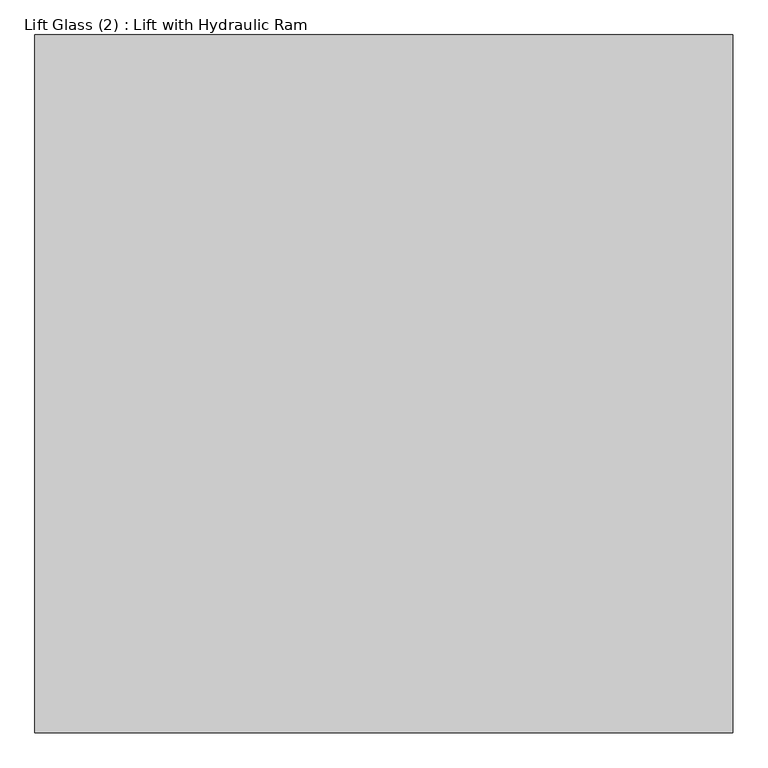
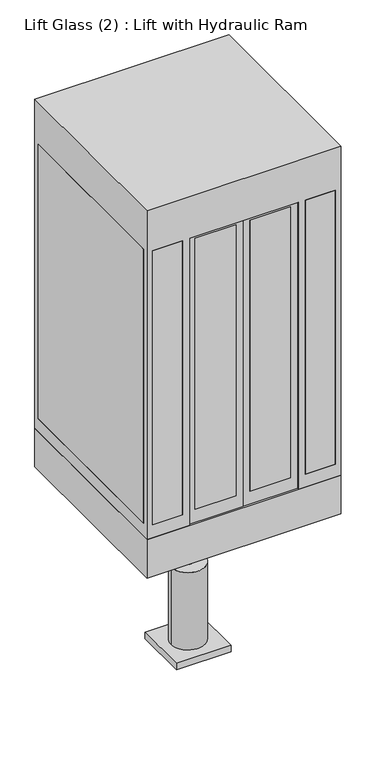
"""IFC4 building model written with IfcOpenShell, lengths in millimetres: proxy geometry, Lift Glass (2) : Lift with Hydraulic Ram."""

from ifc_helpers import new_model, si_unit, point, frame, frame_2d, origin, place, context, project, spatial, polyline, circle_curve, trimmed, segment, composite_curve, outline, extrude, faceted_brep, source, transform, mapped, element, save


def lift_glass_2_lift_with_hydraulic_ram_a28bd677(model_context):
    return source(origin(), model_context, "Body", "SolidModel", [
        extrude(outline(composite_curve([segment(trimmed(circle_curve(frame_2d((34.4858536, 51.9253128)), 35.0), [point((34.4858536, 86.9253128))], [point((34.4858536, 16.9253128))], False, "CARTESIAN"), True, "CONTINUOUS"), segment(trimmed(circle_curve(frame_2d((34.4858536, 51.9253128)), 35.0), [point((34.4858536, 16.9253128))], [point((34.4858536, 86.9253128))], False, "CARTESIAN"), True, "CONTINUOUS")], self_intersect=False)), frame((0.0, 0.0, -850.0), z_axis=(0.0, 0.0, 1.0), x_axis=(1.0, 0.0, 0.0)), (0.0, 0.0, 1.0), 550.0),
        extrude(outline(composite_curve([segment(trimmed(circle_curve(frame_2d((34.4858536, 51.9253128)), 125.0), [point((-90.5141464, 51.9253128))], [point((159.4858536, 51.9253128))], False, "CARTESIAN"), True, "CONTINUOUS"), segment(trimmed(circle_curve(frame_2d((34.4858536, 51.9253128)), 125.0), [point((159.4858536, 51.9253128))], [point((-90.5141464, 51.9253128))], False, "CARTESIAN"), True, "CONTINUOUS")], self_intersect=False)), frame((0.0, 0.0, -1450.0), z_axis=(0.0, 0.0, 1.0), x_axis=(1.0, 0.0, 0.0)), (0.0, 0.0, 1.0), 600.0),
        extrude(outline(polyline([(234.4858536, -148.0746872), (-165.5141464, -148.0746872), (-165.5141464, 251.9253128), (234.4858536, 251.9253128), (234.4858536, -148.0746872)])), frame((0.0, 0.0, -1500.0), z_axis=(0.0, 0.0, 1.0), x_axis=(1.0, 0.0, 0.0)), (0.0, 0.0, 1.0), 50.0),
        extrude(outline(polyline([(-15.5141464, -648.0746872), (-315.5141464, -648.0746872), (-315.5141464, -636.0746872), (-15.5141464, -636.0746872), (-15.5141464, -648.0746872)])), frame((0.0, 0.0, 100.0), z_axis=(0.0, 0.0, 1.0), x_axis=(1.0, 0.0, 0.0)), (0.0, 0.0, 1.0), 2100.0),
        extrude(outline(polyline([(384.4858536, -648.0746872), (84.4858536, -648.0746872), (84.4858536, -636.0746872), (384.4858536, -636.0746872), (384.4858536, -648.0746872)])), frame((0.0, 0.0, 100.0), z_axis=(0.0, 0.0, 1.0), x_axis=(1.0, 0.0, 0.0)), (0.0, 0.0, 1.0), 2100.0),
        extrude(outline(polyline([(2300.0, 33.4858536), (2300.0, -365.5141464), (0.0, -365.5141464), (0.0, 33.4858536), (2300.0, 33.4858536)]), holes=[polyline([(2200.0, -15.5141464), (100.0, -15.5141464), (100.0, -315.5141464), (2200.0, -315.5141464), (2200.0, -15.5141464)])]), frame((0.0, -648.0746872, 0.0), z_axis=(0.0, 1.0, 0.0), x_axis=(0.0, 0.0, 1.0)), (0.0, 0.0, 1.0), 12.0),
        extrude(outline(polyline([(0.0, 35.4858536), (0.0, 434.4858536), (2300.0, 434.4858536), (2300.0, 35.4858536), (0.0, 35.4858536)]), holes=[polyline([(2200.0, 384.4858536), (100.0, 384.4858536), (100.0, 84.4858536), (2200.0, 84.4858536), (2200.0, 384.4858536)])]), frame((0.0, -648.0746872, 0.0), z_axis=(0.0, 1.0, 0.0), x_axis=(0.0, 0.0, 1.0)), (0.0, 0.0, 1.0), 12.0),
        extrude(outline(polyline([(746.4858536, 763.9253128), (746.4858536, -660.0746872), (-677.5141464, -660.0746872), (-677.5141464, 763.9253128), (746.4858536, 763.9253128)])), frame((0.0, 0.0, -300.0), z_axis=(0.0, 0.0, 1.0), x_axis=(1.0, 0.0, 0.0)), (0.0, 0.0, 1.0), 300.0),
        faceted_brep([(734.4858536, 721.9253128, 100.0), (734.4858536, -618.0746872, 100.0), (746.4858536, -618.0746872, 100.0), (746.4858536, 721.9253128, 100.0), (-665.5141464, -618.0746872, 100.0), (-665.5141464, 721.9253128, 100.0), (-677.5141464, 721.9253128, 100.0), (-677.5141464, -618.0746872, 100.0), (-635.5141464, 751.9253128, 100.0), (704.4858536, 751.9253128, 100.0), (704.4858536, 763.9253128, 100.0), (-635.5141464, 763.9253128, 100.0), (704.4858536, -660.0746872, 100.0), (704.4858536, -648.0746872, 100.0), (484.4858536, -648.0746872, 100.0), (484.4858536, -660.0746872, 100.0), (-635.5141464, -648.0746872, 100.0), (-635.5141464, -660.0746872, 100.0), (-415.5141464, -660.0746872, 100.0), (-415.5141464, -648.0746872, 100.0), (434.4858536, -660.0746872, 0.0), (434.4858536, -648.0746872, 0.0), (734.4858536, -648.0746872, 0.0), (734.4858536, 751.9253128, 0.0), (-665.5141464, 751.9253128, 0.0), (-665.5141464, -648.0746872, 0.0), (-365.5141464, -648.0746872, 0.0), (-365.5141464, -660.0746872, 0.0), (-677.5141464, -660.0746872, 0.0), (-677.5141464, 763.9253128, 0.0), (746.4858536, 763.9253128, 0.0), (746.4858536, -660.0746872, 0.0), (734.4858536, 751.9253128, 2300.0), (734.4858536, -648.0746872, 2300.0), (734.4858536, 721.9253128, 2225.0), (734.4858536, -618.0746872, 2225.0), (746.4858536, 763.9253128, 2550.0), (746.4858536, -660.0746872, 2550.0), (746.4858536, -618.0746872, 2225.0), (746.4858536, 721.9253128, 2225.0), (434.4858536, -660.0746872, 2225.0), (434.4858536, -648.0746872, 2225.0), (-677.5141464, -660.0746872, 2550.0), (-365.5141464, -660.0746872, 2225.0), (-635.5141464, -660.0746872, 2225.0), (-415.5141464, -660.0746872, 2225.0), (704.4858536, -660.0746872, 2225.0), (484.4858536, -660.0746872, 2225.0), (-365.5141464, -648.0746872, 2225.0), (-665.5141464, -648.0746872, 2300.0), (-635.5141464, -648.0746872, 2225.0), (-415.5141464, -648.0746872, 2225.0), (704.4858536, -648.0746872, 2225.0), (484.4858536, -648.0746872, 2225.0), (-665.5141464, 751.9253128, 2300.0), (-665.5141464, -618.0746872, 2225.0), (-665.5141464, 721.9253128, 2225.0), (-677.5141464, 763.9253128, 2550.0), (-677.5141464, 721.9253128, 2225.0), (-677.5141464, -618.0746872, 2225.0), (-635.5141464, 751.9253128, 2225.0), (704.4858536, 751.9253128, 2225.0), (704.4858536, 763.9253128, 2225.0), (-635.5141464, 763.9253128, 2225.0)], [[[0, 1, 2, 3]], [[4, 5, 6, 7]], [[8, 9, 10, 11]], [[12, 13, 14, 15]], [[16, 17, 18, 19]], [[20, 21, 22, 23, 24, 25, 26, 27, 28, 29, 30, 31]], [[32, 23, 22, 33], [1, 0, 34, 35]], [[36, 37, 31, 30], [3, 2, 38, 39]], [[21, 20, 40, 41]], [[31, 37, 42, 28, 27, 43, 40, 20], [17, 44, 45, 18], [46, 12, 15, 47]], [[33, 22, 21, 41, 48, 26, 25, 49], [50, 16, 19, 51], [13, 52, 53, 14]], [[27, 26, 48, 43]], [[24, 54, 49, 25], [5, 4, 55, 56]], [[29, 28, 42, 57], [7, 6, 58, 59]], [[23, 32, 54, 24], [9, 8, 60, 61]], [[36, 30, 29, 57], [11, 10, 62, 63]], [[0, 3, 39, 34]], [[10, 9, 61, 62]], [[13, 12, 46, 52]], [[2, 1, 35, 38]], [[8, 11, 63, 60]], [[6, 5, 56, 58]], [[4, 7, 59, 55]], [[17, 16, 50, 44]], [[35, 34, 39, 38]], [[48, 41, 40, 43]], [[56, 55, 59, 58]], [[63, 62, 61, 60]], [[52, 46, 47, 53]], [[44, 50, 51, 45]], [[51, 19, 18, 45]], [[14, 53, 47, 15]], [[57, 42, 37, 36]], [[32, 33, 49, 54]]]),
        extrude(outline(polyline([(734.4858536, -618.0746872), (734.4858536, 721.9253128), (746.4858536, 721.9253128), (746.4858536, -618.0746872), (734.4858536, -618.0746872)])), frame((0.0, 0.0, 100.0), z_axis=(0.0, 0.0, 1.0), x_axis=(1.0, 0.0, 0.0)), (0.0, 0.0, 1.0), 2125.0),
        extrude(outline(polyline([(-415.5141464, -660.0746872), (-635.5141464, -660.0746872), (-635.5141464, -648.0746872), (-415.5141464, -648.0746872), (-415.5141464, -660.0746872)])), frame((0.0, 0.0, 100.0), z_axis=(0.0, 0.0, 1.0), x_axis=(1.0, 0.0, 0.0)), (0.0, 0.0, 1.0), 2125.0),
        extrude(outline(polyline([(704.4858536, -660.0746872), (484.4858536, -660.0746872), (484.4858536, -648.0746872), (704.4858536, -648.0746872), (704.4858536, -660.0746872)])), frame((0.0, 0.0, 100.0), z_axis=(0.0, 0.0, 1.0), x_axis=(1.0, 0.0, 0.0)), (0.0, 0.0, 1.0), 2125.0),
        extrude(outline(polyline([(-665.5141464, -618.0746872), (-677.5141464, -618.0746872), (-677.5141464, 721.9253128), (-665.5141464, 721.9253128), (-665.5141464, -618.0746872)])), frame((0.0, 0.0, 100.0), z_axis=(0.0, 0.0, 1.0), x_axis=(1.0, 0.0, 0.0)), (0.0, 0.0, 1.0), 2125.0),
        extrude(outline(polyline([(704.4858536, 763.9253128), (704.4858536, 751.9253128), (-635.5141464, 751.9253128), (-635.5141464, 763.9253128), (704.4858536, 763.9253128)])), frame((0.0, 0.0, 100.0), z_axis=(0.0, 0.0, 1.0), x_axis=(1.0, 0.0, 0.0)), (0.0, 0.0, 1.0), 2125.0),
    ])


if __name__ == "__main__":
    model = new_model("IFC4")
    model_context = context("Model", 3, world=origin())
    ifc_project = project(units=[si_unit("LENGTHUNIT", "METRE", prefix="MILLI")], contexts=[model_context])
    site = spatial("IfcSite", under=ifc_project)
    building = spatial("IfcBuilding", under=site)
    placement = place(None, origin())
    lift_glass_2_lift_with_hydraulic_ram_shape = lift_glass_2_lift_with_hydraulic_ram_a28bd677(model_context)
    element("IfcBuildingElementProxy", 1, Name="Lift Glass (2) : Lift with Hydraulic Ram", ObjectType="Lift Glass (2) : Lift with Hydraulic Ram", at=placement, inside=building, context=model_context, shape_type="MappedRepresentation", body=[
        mapped(lift_glass_2_lift_with_hydraulic_ram_shape, transform((0.0, 0.0, 0.0), x_axis=(1.0, 0.0, 0.0), y_axis=(0.0, 1.0, 0.0), z_axis=(0.0, 0.0, 1.0))),
    ])
    save(model, "model.ifc")

# Revit data of these elements
# Type "Lift Glass (2) : Lift with Hydraulic Ram"
#   Stile Top Rail = 0' - 3.93701"
#   Stile Shutting = 0' - 1.9685"
#   Stile Hanging Rail = 0' - 1.9685"
#   Stile Bottom = 0' - 3.93701"
#   Skirting Ht = 0' - 3.93701"
#   Hoistway Depth = 5' - 10.86614"
#   Hoistway Width = 6' - 2.80315"
#   Roof Thickness = 0' - 9.84252"
#   Lift Car Width = 4' - 7.11811"
#   Lift Rise = 4' - 11.05512"
#   Lift Height = 7' - 6.55118"
#   Lift Car Depth = 4' - 7.11811"
#   Glazing Thickness = 0' - 0.47244"
#   Floor Thickness = 0' - 11.81102"
#   Floor Offset = 0' - 0.47244"
#   Door Opening = 2' - 7.49606"
#   Door Offset = 0' - 0.98425"
#   Cornice Ht = 0' - 2.95276"
#   Vis - Hydraulic Ram = yes
#   Vis - Hoistway Placement Lines = yes
#   Material Solid panel = Stainless Steel
#   Material Lift Car = Stainless Steel
#   Material Glass = Glass
#   Default Elevation = 0
# Element 1 (IfcBuildingElementProxy, "Lift Glass (2) : Lift with Hydraulic Ram")
#   Materials on its faces: "Stainless Steel", "Glass", "Paint - Green"
# Materials
#   "Stainless Steel": class "Metal", colour RGB 0 0 0, transparency 0, Description = "Stainless Steel 18/8", Cost = 0
#   "Glass": class "Glass", colour RGB 0 128 192, transparency 0.75, Description = "Soda Lime Glass", Cost = 0
#   "Paint - Green": colour RGB 0 128 64, transparency 0
